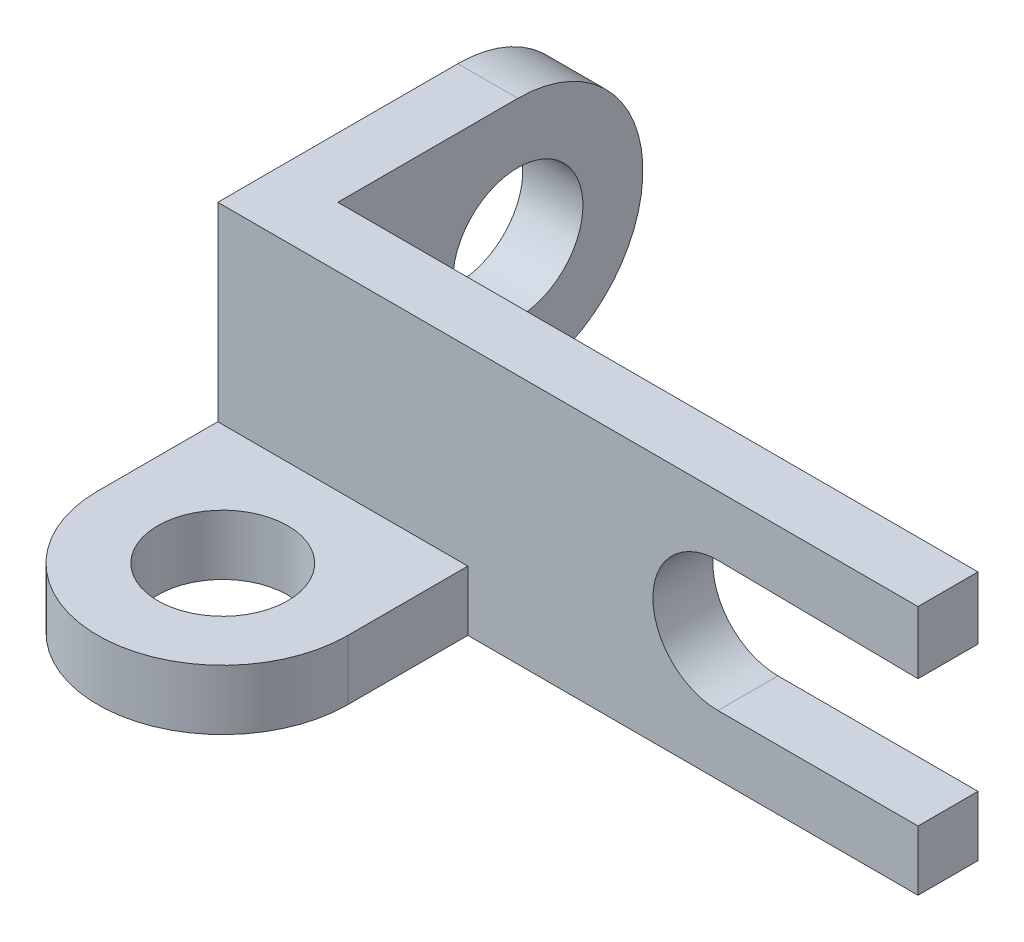
ISO-10303-21;
HEADER;
FILE_DESCRIPTION(('STEP AP214'),'2;1');
FILE_NAME('part.step','',(''),(''),'','','');
FILE_SCHEMA(('AUTOMOTIVE_DESIGN { 1 0 10303 214 1 1 1 1 }'));
ENDSEC;
DATA;
#1=APPLICATION_CONTEXT('core data for automotive mechanical design processes');
#2=APPLICATION_PROTOCOL_DEFINITION('international standard','automotive_design',2000,#1);
#3=PRODUCT_CONTEXT('',#1,'mechanical');
#4=PRODUCT('Part','Part','',(#3));
#5=PRODUCT_RELATED_PRODUCT_CATEGORY('part','',(#4));
#6=PRODUCT_DEFINITION_FORMATION('','',#4);
#7=PRODUCT_DEFINITION_CONTEXT('part definition',#1,'design');
#8=PRODUCT_DEFINITION('design','',#6,#7);
#9=PRODUCT_DEFINITION_SHAPE('','',#8);
#10=(LENGTH_UNIT() NAMED_UNIT(*) SI_UNIT(.MILLI.,.METRE.));
#11=(NAMED_UNIT(*) PLANE_ANGLE_UNIT() SI_UNIT($,.RADIAN.));
#12=(NAMED_UNIT(*) SI_UNIT($,.STERADIAN.) SOLID_ANGLE_UNIT());
#13=UNCERTAINTY_MEASURE_WITH_UNIT(LENGTH_MEASURE(1.E-05),#10,'distance_accuracy_value','');
#14=(GEOMETRIC_REPRESENTATION_CONTEXT(3) GLOBAL_UNCERTAINTY_ASSIGNED_CONTEXT((#13)) GLOBAL_UNIT_ASSIGNED_CONTEXT((#10,
#11,#12)) REPRESENTATION_CONTEXT('',''));
#15=CARTESIAN_POINT('',(0.,0.,0.));
#16=DIRECTION('',(0.,0.,1.));
#17=DIRECTION('',(1.,0.,0.));
#18=AXIS2_PLACEMENT_3D('',#15,#16,#17);
#19=CARTESIAN_POINT('',(0.,0.,0.));
#20=DIRECTION('',(0.,0.,1.));
#21=DIRECTION('',(1.,0.,0.));
#22=AXIS2_PLACEMENT_3D('',#19,#20,#21);
#23=PLANE('',#22);
#24=DIRECTION('',(0.,-1.,0.));
#25=VECTOR('',#24,1.);
#26=CARTESIAN_POINT('',(34.5593869731801,0.,0.));
#27=LINE('',#26,#25);
#28=CARTESIAN_POINT('',(34.5593869731801,6.,0.));
#29=VERTEX_POINT('',#28);
#30=CARTESIAN_POINT('',(34.5593869731801,0.,0.));
#31=VERTEX_POINT('',#30);
#32=EDGE_CURVE('E221',#29,#31,#27,.T.);
#33=ORIENTED_EDGE('',*,*,#32,.T.);
#34=DIRECTION('',(1.,0.,0.));
#35=VECTOR('',#34,1.);
#36=CARTESIAN_POINT('',(0.,0.,0.));
#37=LINE('',#36,#35);
#38=CARTESIAN_POINT('',(-29.4406130268199,0.,0.));
#39=VERTEX_POINT('',#38);
#40=EDGE_CURVE('E225',#39,#31,#37,.T.);
#41=ORIENTED_EDGE('',*,*,#40,.F.);
#42=DIRECTION('',(0.,-1.,0.));
#43=VECTOR('',#42,1.);
#44=CARTESIAN_POINT('',(-29.4406130268199,0.,0.));
#45=LINE('',#44,#43);
#46=CARTESIAN_POINT('',(-29.4406130268199,25.,0.));
#47=VERTEX_POINT('',#46);
#48=EDGE_CURVE('E248',#47,#39,#45,.T.);
#49=ORIENTED_EDGE('',*,*,#48,.F.);
#50=DIRECTION('',(1.,0.,0.));
#51=VECTOR('',#50,1.);
#52=CARTESIAN_POINT('',(0.,25.,0.));
#53=LINE('',#52,#51);
#54=CARTESIAN_POINT('',(34.5593869731801,25.,0.));
#55=VERTEX_POINT('',#54);
#56=EDGE_CURVE('E219',#47,#55,#53,.T.);
#57=ORIENTED_EDGE('',*,*,#56,.T.);
#58=DIRECTION('',(0.,1.,0.));
#59=VECTOR('',#58,1.);
#60=CARTESIAN_POINT('',(34.5593869731801,0.,0.));
#61=LINE('',#60,#59);
#62=CARTESIAN_POINT('',(34.5593869731801,18.7500000000001,0.));
#63=VERTEX_POINT('',#62);
#64=EDGE_CURVE('E220',#63,#55,#61,.T.);
#65=ORIENTED_EDGE('',*,*,#64,.F.);
#66=DIRECTION('',(0.999921884154082,-0.0124990235519205,0.));
#67=VECTOR('',#66,1.);
#68=CARTESIAN_POINT('',(0.239737445238634,19.1789956190992,0.));
#69=LINE('',#68,#67);
#70=CARTESIAN_POINT('',(14.7218615865216,18.9979690673332,0.));
#71=VERTEX_POINT('',#70);
#72=EDGE_CURVE('E214',#71,#63,#69,.T.);
#73=ORIENTED_EDGE('',*,*,#72,.F.);
#74=CARTESIAN_POINT('',(14.5593869731801,12.5,0.));
#75=DIRECTION('',(0.,0.,1.));
#76=DIRECTION('',(1.,0.,0.));
#77=AXIS2_PLACEMENT_3D('',#74,#75,#76);
#78=CIRCLE('',#77,6.5);
#79=CARTESIAN_POINT('',(14.5593869731801,6.,0.));
#80=VERTEX_POINT('',#79);
#81=EDGE_CURVE('E188',#71,#80,#78,.T.);
#82=ORIENTED_EDGE('',*,*,#81,.T.);
#83=DIRECTION('',(1.,0.,0.));
#84=VECTOR('',#83,1.);
#85=CARTESIAN_POINT('',(0.,6.,0.));
#86=LINE('',#85,#84);
#87=EDGE_CURVE('E198',#80,#29,#86,.T.);
#88=ORIENTED_EDGE('',*,*,#87,.T.);
#89=EDGE_LOOP('',(#33,#41,#49,#57,#65,#73,#82,#88));
#90=FACE_BOUND('',#89,.T.);
#91=ADVANCED_FACE('F41',(#90),#23,.F.);
#92=CARTESIAN_POINT('',(14.5593869731801,12.5,6.));
#93=DIRECTION('',(0.,0.,-1.));
#94=DIRECTION('',(-1.,0.,0.));
#95=AXIS2_PLACEMENT_3D('',#92,#93,#94);
#96=CYLINDRICAL_SURFACE('',#95,6.5);
#97=ORIENTED_EDGE('',*,*,#81,.F.);
#98=DIRECTION('',(0.,0.,-1.));
#99=VECTOR('',#98,1.);
#100=CARTESIAN_POINT('',(14.7218615865216,18.9979690673332,6.));
#101=LINE('',#100,#99);
#102=CARTESIAN_POINT('',(14.7218615865216,18.9979690673332,6.));
#103=VERTEX_POINT('',#102);
#104=EDGE_CURVE('E243',#103,#71,#101,.T.);
#105=ORIENTED_EDGE('',*,*,#104,.F.);
#106=CARTESIAN_POINT('',(14.5593869731801,12.5,6.));
#107=DIRECTION('',(0.,0.,1.));
#108=DIRECTION('',(1.,0.,0.));
#109=AXIS2_PLACEMENT_3D('',#106,#107,#108);
#110=CIRCLE('',#109,6.5);
#111=CARTESIAN_POINT('',(14.5593869731801,6.,6.));
#112=VERTEX_POINT('',#111);
#113=EDGE_CURVE('E194',#103,#112,#110,.T.);
#114=ORIENTED_EDGE('',*,*,#113,.T.);
#115=DIRECTION('',(0.,0.,-1.));
#116=VECTOR('',#115,1.);
#117=CARTESIAN_POINT('',(14.5593869731801,6.,6.));
#118=LINE('',#117,#116);
#119=EDGE_CURVE('E215',#112,#80,#118,.T.);
#120=ORIENTED_EDGE('',*,*,#119,.T.);
#121=EDGE_LOOP('',(#97,#105,#114,#120));
#122=FACE_BOUND('',#121,.T.);
#123=ADVANCED_FACE('F43',(#122),#96,.F.);
#124=CARTESIAN_POINT('',(0.239737445238634,19.1789956190992,6.));
#125=DIRECTION('',(0.0124990235519205,0.999921884154082,0.));
#126=DIRECTION('',(-0.999921884154082,0.0124990235519205,0.));
#127=AXIS2_PLACEMENT_3D('',#124,#125,#126);
#128=PLANE('',#127);
#129=ORIENTED_EDGE('',*,*,#72,.T.);
#130=DIRECTION('',(0.,0.,-1.));
#131=VECTOR('',#130,1.);
#132=CARTESIAN_POINT('',(34.5593869731801,18.7500000000001,6.));
#133=LINE('',#132,#131);
#134=CARTESIAN_POINT('',(34.5593869731801,18.7500000000001,6.));
#135=VERTEX_POINT('',#134);
#136=EDGE_CURVE('E241',#135,#63,#133,.T.);
#137=ORIENTED_EDGE('',*,*,#136,.F.);
#138=DIRECTION('',(0.999921884154082,-0.0124990235519205,0.));
#139=VECTOR('',#138,1.);
#140=CARTESIAN_POINT('',(0.239737445238634,19.1789956190992,6.));
#141=LINE('',#140,#139);
#142=EDGE_CURVE('E191',#103,#135,#141,.T.);
#143=ORIENTED_EDGE('',*,*,#142,.F.);
#144=ORIENTED_EDGE('',*,*,#104,.T.);
#145=EDGE_LOOP('',(#129,#137,#143,#144));
#146=FACE_BOUND('',#145,.T.);
#147=ADVANCED_FACE('F280',(#146),#128,.F.);
#148=CARTESIAN_POINT('',(34.5593869731801,0.,6.));
#149=DIRECTION('',(-1.,0.,0.));
#150=DIRECTION('',(0.,0.,1.));
#151=AXIS2_PLACEMENT_3D('',#148,#149,#150);
#152=PLANE('',#151);
#153=ORIENTED_EDGE('',*,*,#64,.T.);
#154=DIRECTION('',(0.,0.,-1.));
#155=VECTOR('',#154,1.);
#156=CARTESIAN_POINT('',(34.5593869731801,25.,6.));
#157=LINE('',#156,#155);
#158=CARTESIAN_POINT('',(34.5593869731801,25.,6.));
#159=VERTEX_POINT('',#158);
#160=EDGE_CURVE('E236',#159,#55,#157,.T.);
#161=ORIENTED_EDGE('',*,*,#160,.F.);
#162=DIRECTION('',(0.,1.,0.));
#163=VECTOR('',#162,1.);
#164=CARTESIAN_POINT('',(34.5593869731801,0.,6.));
#165=LINE('',#164,#163);
#166=EDGE_CURVE('E196',#135,#159,#165,.T.);
#167=ORIENTED_EDGE('',*,*,#166,.F.);
#168=ORIENTED_EDGE('',*,*,#136,.T.);
#169=EDGE_LOOP('',(#153,#161,#167,#168));
#170=FACE_BOUND('',#169,.T.);
#171=ADVANCED_FACE('F275',(#170),#152,.F.);
#172=CARTESIAN_POINT('',(0.,25.,6.));
#173=DIRECTION('',(0.,1.,0.));
#174=DIRECTION('',(0.,0.,1.));
#175=AXIS2_PLACEMENT_3D('',#172,#173,#174);
#176=PLANE('',#175);
#177=DIRECTION('',(1.,0.,0.));
#178=VECTOR('',#177,1.);
#179=CARTESIAN_POINT('',(0.,25.,6.));
#180=LINE('',#179,#178);
#181=CARTESIAN_POINT('',(-35.4406130268199,25.,6.));
#182=VERTEX_POINT('',#181);
#183=EDGE_CURVE('E203',#182,#159,#180,.T.);
#184=ORIENTED_EDGE('',*,*,#183,.T.);
#185=ORIENTED_EDGE('',*,*,#160,.T.);
#186=ORIENTED_EDGE('',*,*,#56,.F.);
#187=DIRECTION('',(0.,0.,-1.));
#188=VECTOR('',#187,1.);
#189=CARTESIAN_POINT('',(-29.4406130268199,25.,6.));
#190=LINE('',#189,#188);
#191=CARTESIAN_POINT('',(-29.4406130268199,25.,-18.));
#192=VERTEX_POINT('',#191);
#193=EDGE_CURVE('E185',#47,#192,#190,.T.);
#194=ORIENTED_EDGE('',*,*,#193,.T.);
#195=DIRECTION('',(-1.,0.,0.));
#196=VECTOR('',#195,1.);
#197=CARTESIAN_POINT('',(-29.4406130268199,25.,-18.));
#198=LINE('',#197,#196);
#199=CARTESIAN_POINT('',(-35.4406130268199,25.,-18.));
#200=VERTEX_POINT('',#199);
#201=EDGE_CURVE('E186',#192,#200,#198,.T.);
#202=ORIENTED_EDGE('',*,*,#201,.T.);
#203=DIRECTION('',(0.,0.,-1.));
#204=VECTOR('',#203,1.);
#205=CARTESIAN_POINT('',(-35.4406130268199,25.,6.));
#206=LINE('',#205,#204);
#207=EDGE_CURVE('E237',#182,#200,#206,.T.);
#208=ORIENTED_EDGE('',*,*,#207,.F.);
#209=EDGE_LOOP('',(#184,#185,#186,#194,#202,#208));
#210=FACE_BOUND('',#209,.T.);
#211=ADVANCED_FACE('F266',(#210),#176,.T.);
#212=CARTESIAN_POINT('',(-35.4406130268199,0.,6.));
#213=DIRECTION('',(-1.,0.,0.));
#214=DIRECTION('',(0.,0.,1.));
#215=AXIS2_PLACEMENT_3D('',#212,#213,#214);
#216=PLANE('',#215);
#217=CARTESIAN_POINT('',(-35.4406130268199,12.5,-18.));
#218=DIRECTION('',(-1.,0.,0.));
#219=DIRECTION('',(0.,0.,1.));
#220=AXIS2_PLACEMENT_3D('',#217,#218,#219);
#221=CIRCLE('',#220,12.5);
#222=CARTESIAN_POINT('',(-35.4406130268199,0.,-18.));
#223=VERTEX_POINT('',#222);
#224=EDGE_CURVE('E174',#200,#223,#221,.T.);
#225=ORIENTED_EDGE('',*,*,#224,.T.);
#226=DIRECTION('',(0.,0.,-1.));
#227=VECTOR('',#226,1.);
#228=CARTESIAN_POINT('',(-35.4406130268199,0.,6.));
#229=LINE('',#228,#227);
#230=CARTESIAN_POINT('',(-35.4406130268199,0.,18.));
#231=VERTEX_POINT('',#230);
#232=EDGE_CURVE('E140',#231,#223,#229,.T.);
#233=ORIENTED_EDGE('',*,*,#232,.F.);
#234=DIRECTION('',(0.,-1.,0.));
#235=VECTOR('',#234,1.);
#236=CARTESIAN_POINT('',(-35.4406130268199,6.,18.));
#237=LINE('',#236,#235);
#238=CARTESIAN_POINT('',(-35.4406130268199,6.,18.));
#239=VERTEX_POINT('',#238);
#240=EDGE_CURVE('E134',#239,#231,#237,.T.);
#241=ORIENTED_EDGE('',*,*,#240,.F.);
#242=DIRECTION('',(0.,0.,-1.));
#243=VECTOR('',#242,1.);
#244=CARTESIAN_POINT('',(-35.4406130268199,6.,18.));
#245=LINE('',#244,#243);
#246=CARTESIAN_POINT('',(-35.4406130268199,6.,6.));
#247=VERTEX_POINT('',#246);
#248=EDGE_CURVE('E137',#239,#247,#245,.T.);
#249=ORIENTED_EDGE('',*,*,#248,.T.);
#250=DIRECTION('',(0.,1.,0.));
#251=VECTOR('',#250,1.);
#252=CARTESIAN_POINT('',(-35.4406130268199,0.,6.));
#253=LINE('',#252,#251);
#254=EDGE_CURVE('E56',#247,#182,#253,.T.);
#255=ORIENTED_EDGE('',*,*,#254,.T.);
#256=ORIENTED_EDGE('',*,*,#207,.T.);
#257=EDGE_LOOP('',(#225,#233,#241,#249,#255,#256));
#258=FACE_BOUND('',#257,.T.);
#259=CARTESIAN_POINT('',(-35.4406130268199,12.5,-18.));
#260=DIRECTION('',(-1.,0.,0.));
#261=DIRECTION('',(0.,0.,1.));
#262=AXIS2_PLACEMENT_3D('',#259,#260,#261);
#263=CIRCLE('',#262,6.5);
#264=CARTESIAN_POINT('',(-35.4406130268199,12.5,-11.5));
#265=VERTEX_POINT('',#264);
#266=EDGE_CURVE('E169',#265,#265,#263,.T.);
#267=ORIENTED_EDGE('',*,*,#266,.F.);
#268=EDGE_LOOP('',(#267));
#269=FACE_BOUND('',#268,.T.);
#270=ADVANCED_FACE('F138',(#258,#269),#216,.T.);
#271=CARTESIAN_POINT('',(0.,0.,6.));
#272=DIRECTION('',(0.,1.,0.));
#273=DIRECTION('',(0.,0.,1.));
#274=AXIS2_PLACEMENT_3D('',#271,#272,#273);
#275=PLANE('',#274);
#276=DIRECTION('',(0.,0.,1.));
#277=VECTOR('',#276,1.);
#278=CARTESIAN_POINT('',(-29.4406130268199,0.,-18.));
#279=LINE('',#278,#277);
#280=CARTESIAN_POINT('',(-29.4406130268199,0.,-18.));
#281=VERTEX_POINT('',#280);
#282=EDGE_CURVE('E180',#281,#39,#279,.T.);
#283=ORIENTED_EDGE('',*,*,#282,.T.);
#284=ORIENTED_EDGE('',*,*,#40,.T.);
#285=DIRECTION('',(0.,0.,-1.));
#286=VECTOR('',#285,1.);
#287=CARTESIAN_POINT('',(34.5593869731801,0.,6.));
#288=LINE('',#287,#286);
#289=CARTESIAN_POINT('',(34.5593869731801,0.,6.));
#290=VERTEX_POINT('',#289);
#291=EDGE_CURVE('E234',#290,#31,#288,.T.);
#292=ORIENTED_EDGE('',*,*,#291,.F.);
#293=DIRECTION('',(1.,0.,0.));
#294=VECTOR('',#293,1.);
#295=CARTESIAN_POINT('',(0.,0.,6.));
#296=LINE('',#295,#294);
#297=CARTESIAN_POINT('',(-10.4406130268199,0.,6.));
#298=VERTEX_POINT('',#297);
#299=EDGE_CURVE('E204',#298,#290,#296,.T.);
#300=ORIENTED_EDGE('',*,*,#299,.F.);
#301=DIRECTION('',(0.,0.,1.));
#302=VECTOR('',#301,1.);
#303=CARTESIAN_POINT('',(-10.4406130268199,0.,0.));
#304=LINE('',#303,#302);
#305=CARTESIAN_POINT('',(-10.4406130268199,0.,18.));
#306=VERTEX_POINT('',#305);
#307=EDGE_CURVE('E160',#298,#306,#304,.T.);
#308=ORIENTED_EDGE('',*,*,#307,.T.);
#309=CARTESIAN_POINT('',(-22.9406130268199,0.,18.));
#310=DIRECTION('',(0.,-1.,0.));
#311=DIRECTION('',(0.,0.,-1.));
#312=AXIS2_PLACEMENT_3D('',#309,#310,#311);
#313=CIRCLE('',#312,12.5);
#314=EDGE_CURVE('E157',#306,#231,#313,.T.);
#315=ORIENTED_EDGE('',*,*,#314,.T.);
#316=ORIENTED_EDGE('',*,*,#232,.T.);
#317=DIRECTION('',(-1.,0.,0.));
#318=VECTOR('',#317,1.);
#319=CARTESIAN_POINT('',(-29.4406130268199,0.,-18.));
#320=LINE('',#319,#318);
#321=EDGE_CURVE('E184',#281,#223,#320,.T.);
#322=ORIENTED_EDGE('',*,*,#321,.F.);
#323=EDGE_LOOP('',(#283,#284,#292,#300,#308,#315,#316,#322));
#324=FACE_BOUND('',#323,.T.);
#325=CARTESIAN_POINT('',(-22.9406130268199,0.,18.));
#326=DIRECTION('',(0.,-1.,0.));
#327=DIRECTION('',(0.,0.,-1.));
#328=AXIS2_PLACEMENT_3D('',#325,#326,#327);
#329=CIRCLE('',#328,6.5);
#330=CARTESIAN_POINT('',(-22.9406130268199,0.,11.5));
#331=VERTEX_POINT('',#330);
#332=EDGE_CURVE('E165',#331,#331,#329,.T.);
#333=ORIENTED_EDGE('',*,*,#332,.F.);
#334=EDGE_LOOP('',(#333));
#335=FACE_BOUND('',#334,.T.);
#336=ADVANCED_FACE('F256',(#324,#335),#275,.F.);
#337=CARTESIAN_POINT('',(34.5593869731801,0.,6.));
#338=DIRECTION('',(1.,0.,0.));
#339=DIRECTION('',(0.,0.,-1.));
#340=AXIS2_PLACEMENT_3D('',#337,#338,#339);
#341=PLANE('',#340);
#342=ORIENTED_EDGE('',*,*,#32,.F.);
#343=DIRECTION('',(0.,0.,-1.));
#344=VECTOR('',#343,1.);
#345=CARTESIAN_POINT('',(34.5593869731801,6.,6.));
#346=LINE('',#345,#344);
#347=CARTESIAN_POINT('',(34.5593869731801,6.,6.));
#348=VERTEX_POINT('',#347);
#349=EDGE_CURVE('E230',#348,#29,#346,.T.);
#350=ORIENTED_EDGE('',*,*,#349,.F.);
#351=DIRECTION('',(0.,-1.,0.));
#352=VECTOR('',#351,1.);
#353=CARTESIAN_POINT('',(34.5593869731801,0.,6.));
#354=LINE('',#353,#352);
#355=EDGE_CURVE('E206',#348,#290,#354,.T.);
#356=ORIENTED_EDGE('',*,*,#355,.T.);
#357=ORIENTED_EDGE('',*,*,#291,.T.);
#358=EDGE_LOOP('',(#342,#350,#356,#357));
#359=FACE_BOUND('',#358,.T.);
#360=ADVANCED_FACE('F288',(#359),#341,.T.);
#361=CARTESIAN_POINT('',(0.,6.,6.));
#362=DIRECTION('',(0.,1.,0.));
#363=DIRECTION('',(0.,0.,1.));
#364=AXIS2_PLACEMENT_3D('',#361,#362,#363);
#365=PLANE('',#364);
#366=ORIENTED_EDGE('',*,*,#87,.F.);
#367=ORIENTED_EDGE('',*,*,#119,.F.);
#368=DIRECTION('',(1.,0.,0.));
#369=VECTOR('',#368,1.);
#370=CARTESIAN_POINT('',(0.,6.,6.));
#371=LINE('',#370,#369);
#372=EDGE_CURVE('E207',#112,#348,#371,.T.);
#373=ORIENTED_EDGE('',*,*,#372,.T.);
#374=ORIENTED_EDGE('',*,*,#349,.T.);
#375=EDGE_LOOP('',(#366,#367,#373,#374));
#376=FACE_BOUND('',#375,.T.);
#377=ADVANCED_FACE('F284',(#376),#365,.T.);
#378=CARTESIAN_POINT('',(0.,0.,6.));
#379=DIRECTION('',(0.,0.,1.));
#380=DIRECTION('',(1.,0.,0.));
#381=AXIS2_PLACEMENT_3D('',#378,#379,#380);
#382=PLANE('',#381);
#383=DIRECTION('',(0.,1.,0.));
#384=VECTOR('',#383,1.);
#385=CARTESIAN_POINT('',(-10.4406130268199,0.,6.));
#386=LINE('',#385,#384);
#387=CARTESIAN_POINT('',(-10.4406130268199,6.,6.));
#388=VERTEX_POINT('',#387);
#389=EDGE_CURVE('E11',#298,#388,#386,.T.);
#390=ORIENTED_EDGE('',*,*,#389,.F.);
#391=ORIENTED_EDGE('',*,*,#299,.T.);
#392=ORIENTED_EDGE('',*,*,#355,.F.);
#393=ORIENTED_EDGE('',*,*,#372,.F.);
#394=ORIENTED_EDGE('',*,*,#113,.F.);
#395=ORIENTED_EDGE('',*,*,#142,.T.);
#396=ORIENTED_EDGE('',*,*,#166,.T.);
#397=ORIENTED_EDGE('',*,*,#183,.F.);
#398=ORIENTED_EDGE('',*,*,#254,.F.);
#399=DIRECTION('',(1.,0.,0.));
#400=VECTOR('',#399,1.);
#401=CARTESIAN_POINT('',(0.,6.,6.));
#402=LINE('',#401,#400);
#403=EDGE_CURVE('E47',#247,#388,#402,.T.);
#404=ORIENTED_EDGE('',*,*,#403,.T.);
#405=EDGE_LOOP('',(#390,#391,#392,#393,#394,#395,#396,#397,#398,#404));
#406=FACE_BOUND('',#405,.T.);
#407=ADVANCED_FACE('F287',(#406),#382,.T.);
#408=CARTESIAN_POINT('',(-29.4406130268199,12.5,-18.));
#409=DIRECTION('',(-1.,0.,0.));
#410=DIRECTION('',(0.,0.,1.));
#411=AXIS2_PLACEMENT_3D('',#408,#409,#410);
#412=PLANE('',#411);
#413=CARTESIAN_POINT('',(-29.4406130268199,12.5,-18.));
#414=DIRECTION('',(-1.,0.,0.));
#415=DIRECTION('',(0.,0.,1.));
#416=AXIS2_PLACEMENT_3D('',#413,#414,#415);
#417=CIRCLE('',#416,6.5);
#418=CARTESIAN_POINT('',(-29.4406130268199,12.5,-11.5));
#419=VERTEX_POINT('',#418);
#420=EDGE_CURVE('E168',#419,#419,#417,.T.);
#421=ORIENTED_EDGE('',*,*,#420,.T.);
#422=EDGE_LOOP('',(#421));
#423=FACE_BOUND('',#422,.T.);
#424=ORIENTED_EDGE('',*,*,#193,.F.);
#425=ORIENTED_EDGE('',*,*,#48,.T.);
#426=ORIENTED_EDGE('',*,*,#282,.F.);
#427=CARTESIAN_POINT('',(-29.4406130268199,12.5,-18.));
#428=DIRECTION('',(-1.,0.,0.));
#429=DIRECTION('',(0.,0.,1.));
#430=AXIS2_PLACEMENT_3D('',#427,#428,#429);
#431=CIRCLE('',#430,12.5);
#432=EDGE_CURVE('E178',#192,#281,#431,.T.);
#433=ORIENTED_EDGE('',*,*,#432,.F.);
#434=EDGE_LOOP('',(#424,#425,#426,#433));
#435=FACE_BOUND('',#434,.T.);
#436=ADVANCED_FACE('F253',(#423,#435),#412,.F.);
#437=CARTESIAN_POINT('',(-29.4406130268199,12.5,-18.));
#438=DIRECTION('',(-1.,0.,0.));
#439=DIRECTION('',(0.,0.,1.));
#440=AXIS2_PLACEMENT_3D('',#437,#438,#439);
#441=CYLINDRICAL_SURFACE('',#440,12.5);
#442=ORIENTED_EDGE('',*,*,#224,.F.);
#443=ORIENTED_EDGE('',*,*,#201,.F.);
#444=ORIENTED_EDGE('',*,*,#432,.T.);
#445=ORIENTED_EDGE('',*,*,#321,.T.);
#446=EDGE_LOOP('',(#442,#443,#444,#445));
#447=FACE_BOUND('',#446,.T.);
#448=ADVANCED_FACE('F265',(#447),#441,.T.);
#449=CARTESIAN_POINT('',(-29.4406130268199,12.5,-18.));
#450=DIRECTION('',(-1.,0.,0.));
#451=DIRECTION('',(0.,0.,1.));
#452=AXIS2_PLACEMENT_3D('',#449,#450,#451);
#453=CYLINDRICAL_SURFACE('',#452,6.5);
#454=ORIENTED_EDGE('',*,*,#420,.F.);
#455=EDGE_LOOP('',(#454));
#456=FACE_BOUND('',#455,.T.);
#457=ORIENTED_EDGE('',*,*,#266,.T.);
#458=EDGE_LOOP('',(#457));
#459=FACE_BOUND('',#458,.T.);
#460=ADVANCED_FACE('F298',(#456,#459),#453,.F.);
#461=CARTESIAN_POINT('',(-22.9406130268199,6.,18.));
#462=DIRECTION('',(0.,-1.,0.));
#463=DIRECTION('',(0.,0.,-1.));
#464=AXIS2_PLACEMENT_3D('',#461,#462,#463);
#465=CYLINDRICAL_SURFACE('',#464,12.5);
#466=ORIENTED_EDGE('',*,*,#314,.F.);
#467=DIRECTION('',(0.,-1.,0.));
#468=VECTOR('',#467,1.);
#469=CARTESIAN_POINT('',(-10.4406130268199,6.,18.));
#470=LINE('',#469,#468);
#471=CARTESIAN_POINT('',(-10.4406130268199,6.,18.));
#472=VERTEX_POINT('',#471);
#473=EDGE_CURVE('E145',#472,#306,#470,.T.);
#474=ORIENTED_EDGE('',*,*,#473,.F.);
#475=CARTESIAN_POINT('',(-22.9406130268199,6.,18.));
#476=DIRECTION('',(0.,-1.,0.));
#477=DIRECTION('',(0.,0.,-1.));
#478=AXIS2_PLACEMENT_3D('',#475,#476,#477);
#479=CIRCLE('',#478,12.5);
#480=EDGE_CURVE('E155',#472,#239,#479,.T.);
#481=ORIENTED_EDGE('',*,*,#480,.T.);
#482=ORIENTED_EDGE('',*,*,#240,.T.);
#483=EDGE_LOOP('',(#466,#474,#481,#482));
#484=FACE_BOUND('',#483,.T.);
#485=ADVANCED_FACE('F154',(#484),#465,.T.);
#486=CARTESIAN_POINT('',(-10.4406130268199,6.,0.));
#487=DIRECTION('',(1.,0.,0.));
#488=DIRECTION('',(0.,0.,-1.));
#489=AXIS2_PLACEMENT_3D('',#486,#487,#488);
#490=PLANE('',#489);
#491=ORIENTED_EDGE('',*,*,#307,.F.);
#492=ORIENTED_EDGE('',*,*,#389,.T.);
#493=DIRECTION('',(0.,0.,1.));
#494=VECTOR('',#493,1.);
#495=CARTESIAN_POINT('',(-10.4406130268199,6.,0.));
#496=LINE('',#495,#494);
#497=EDGE_CURVE('E144',#388,#472,#496,.T.);
#498=ORIENTED_EDGE('',*,*,#497,.T.);
#499=ORIENTED_EDGE('',*,*,#473,.T.);
#500=EDGE_LOOP('',(#491,#492,#498,#499));
#501=FACE_BOUND('',#500,.T.);
#502=ADVANCED_FACE('F286',(#501),#490,.T.);
#503=CARTESIAN_POINT('',(-22.9406130268199,6.,18.));
#504=DIRECTION('',(0.,-1.,0.));
#505=DIRECTION('',(0.,0.,-1.));
#506=AXIS2_PLACEMENT_3D('',#503,#504,#505);
#507=PLANE('',#506);
#508=ORIENTED_EDGE('',*,*,#403,.F.);
#509=ORIENTED_EDGE('',*,*,#248,.F.);
#510=ORIENTED_EDGE('',*,*,#480,.F.);
#511=ORIENTED_EDGE('',*,*,#497,.F.);
#512=EDGE_LOOP('',(#508,#509,#510,#511));
#513=FACE_BOUND('',#512,.T.);
#514=CARTESIAN_POINT('',(-22.9406130268199,6.,18.));
#515=DIRECTION('',(0.,-1.,0.));
#516=DIRECTION('',(0.,0.,-1.));
#517=AXIS2_PLACEMENT_3D('',#514,#515,#516);
#518=CIRCLE('',#517,6.5);
#519=CARTESIAN_POINT('',(-22.9406130268199,6.,11.5));
#520=VERTEX_POINT('',#519);
#521=EDGE_CURVE('E167',#520,#520,#518,.T.);
#522=ORIENTED_EDGE('',*,*,#521,.T.);
#523=EDGE_LOOP('',(#522));
#524=FACE_BOUND('',#523,.T.);
#525=ADVANCED_FACE('F149',(#513,#524),#507,.F.);
#526=CARTESIAN_POINT('',(-22.9406130268199,6.,18.));
#527=DIRECTION('',(0.,-1.,0.));
#528=DIRECTION('',(0.,0.,-1.));
#529=AXIS2_PLACEMENT_3D('',#526,#527,#528);
#530=CYLINDRICAL_SURFACE('',#529,6.5);
#531=ORIENTED_EDGE('',*,*,#521,.F.);
#532=EDGE_LOOP('',(#531));
#533=FACE_BOUND('',#532,.T.);
#534=ORIENTED_EDGE('',*,*,#332,.T.);
#535=EDGE_LOOP('',(#534));
#536=FACE_BOUND('',#535,.T.);
#537=ADVANCED_FACE('F297',(#533,#536),#530,.F.);
#538=CLOSED_SHELL('',(#91,#123,#147,#171,#211,#270,#336,#360,#377,#407,#436,#448,#460,#485,#502,
#525,#537));
#539=MANIFOLD_SOLID_BREP('B2',#538);
#540=ADVANCED_BREP_SHAPE_REPRESENTATION('',(#18,#539),#14);
#541=SHAPE_DEFINITION_REPRESENTATION(#9,#540);
ENDSEC;
END-ISO-10303-21;
